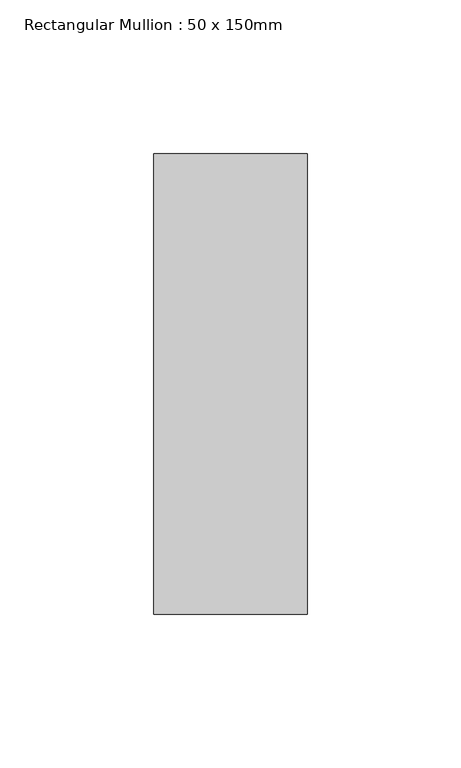
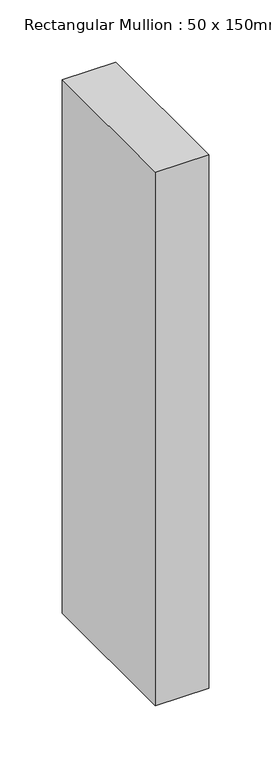
"""IFC4 building model written with IfcOpenShell, lengths in millimetres: member geometry, Rectangular Mullion : 50 x 150mm."""

from ifc_helpers import new_model, si_unit, frame, origin, place, context, project, spatial, polyline, outline, extrude, source, transform, mapped, element, save


def rectangular_mullion_50_x_150mm_8a69f4a4(model_context):
    return source(origin(), model_context, "Body", "SweptSolid", [
        extrude(outline(polyline([(25.0, 75.0), (25.0, -75.0), (-25.0, -75.0), (-25.0, 75.0), (25.0, 75.0)])), frame((0.0, 0.0, -525.0), z_axis=(0.0, 0.0, 1.0), x_axis=(1.0, 0.0, 0.0)), (0.0, 0.0, 1.0), 525.0),
    ])


if __name__ == "__main__":
    model = new_model("IFC4")
    model_context = context("Model", 3, world=origin())
    ifc_project = project(units=[si_unit("LENGTHUNIT", "METRE", prefix="MILLI")], contexts=[model_context])
    site = spatial("IfcSite", under=ifc_project)
    building = spatial("IfcBuilding", under=site)
    placement = place(None, origin())
    rectangular_mullion_50_x_150mm_shape = rectangular_mullion_50_x_150mm_8a69f4a4(model_context)
    element("IfcMember", 1, ObjectType="Rectangular Mullion : 50 x 150mm", at=placement, inside=building, context=model_context, shape_type="MappedRepresentation", body=[
        mapped(rectangular_mullion_50_x_150mm_shape, transform((0.0, 0.0, 0.0), x_axis=(1.0, 0.0, 0.0), y_axis=(0.0, 1.0, 0.0), z_axis=(0.0, 0.0, 1.0))),
    ])
    save(model, "model.ifc")

# Revit data of these elements
# Type "Rectangular Mullion : 50 x 150mm"
#   built-in parameter 1007304 = 0.492126 (stored number, unit not read)
#   built-in parameter 1007301 = 0.082021 (stored number, unit not read)
#   built-in parameter 1007300 = 0.082021 (stored number, unit not read)
# Element 1 (IfcMember, "Rectangular Mullion : 50 x 150mm")
#   Materials on its faces: "Aluminium"
# Materials
#   "Aluminium": class "Metal", colour RGB 247 247 247, transparency 0, Description = "Aluminium 6061", Cost = 0
